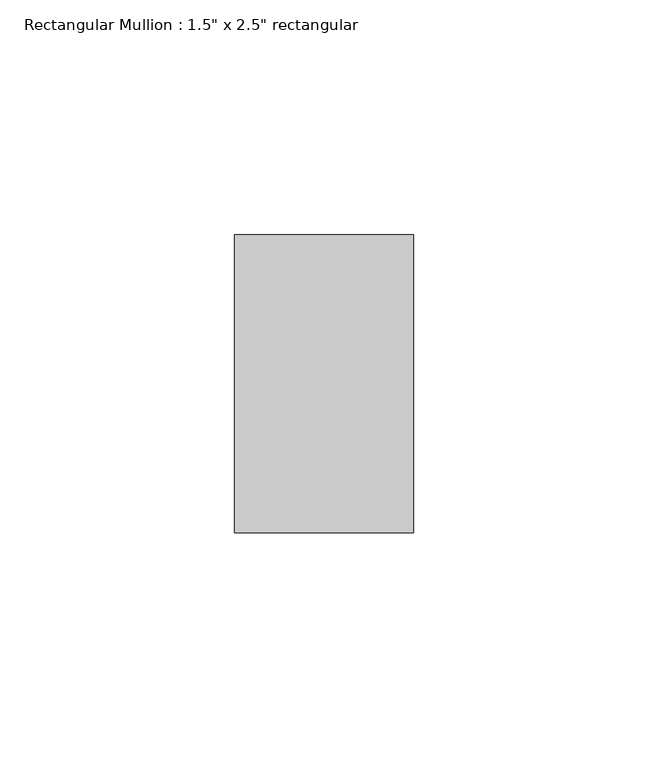
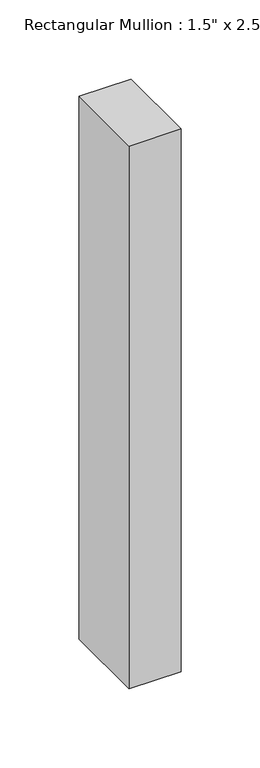
"""IFC4 building model written with IfcOpenShell, lengths in millimetres: member geometry."""

from ifc_helpers import new_model, si_unit, frame, origin, place, context, project, spatial, polyline, outline, extrude, source, transform, mapped, element, save


def member_8587bb6c(model_context):
    return source(origin(), model_context, "Body", "SweptSolid", [
        extrude(outline(polyline([(0.0, 31.75), (0.0, -31.75), (-38.1, -31.75), (-38.1, 31.75), (0.0, 31.75)])), frame((0.0, 0.0, -419.1), z_axis=(0.0, 0.0, 1.0), x_axis=(1.0, 0.0, 0.0)), (0.0, 0.0, 1.0), 419.1),
    ])


if __name__ == "__main__":
    model = new_model("IFC4")
    model_context = context("Model", 3, world=origin())
    ifc_project = project(units=[si_unit("LENGTHUNIT", "METRE", prefix="MILLI")], contexts=[model_context])
    site = spatial("IfcSite", under=ifc_project)
    building = spatial("IfcBuilding", under=site)
    placement = place(None, origin())
    member_shape = member_8587bb6c(model_context)
    element("IfcMember", 1, ObjectType="Rectangular Mullion : 1.5\" x 2.5\" rectangular", at=placement, inside=building, context=model_context, shape_type="MappedRepresentation", body=[
        mapped(member_shape, transform((0.0, 0.0, 0.0), x_axis=(1.0, 0.0, 0.0), y_axis=(0.0, 1.0, 0.0), z_axis=(0.0, 0.0, 1.0))),
    ])
    save(model, "model.ifc")

# Revit data of these elements
# Type "Rectangular Mullion : 1.5\" x 2.5\" rectangular"
#   built-in parameter 1007304 = 0.208333 (stored number, unit not read)
#   built-in parameter 1007301 = 0.0625 (stored number, unit not read)
#   built-in parameter 1007300 = 0.0625 (stored number, unit not read)
# Element 1 (IfcMember, "Rectangular Mullion : 1.5\" x 2.5\" rectangular")
#   Materials on its faces: "Aluminum"
# Materials
#   "Aluminum": class "Metal", colour RGB 247 247 247, transparency 0, Description = "Aluminum 6061", Cost = 0
